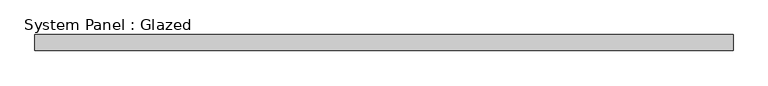
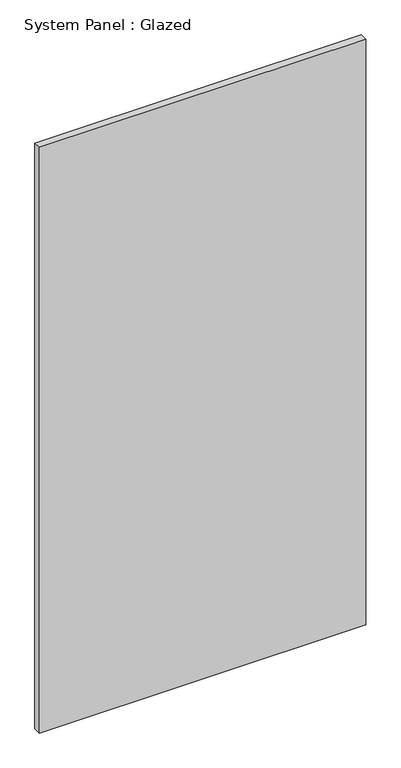
"""IFC4 building model written with IfcOpenShell, lengths in millimetres: plate geometry, System Panel : Glazed."""

from ifc_helpers import new_model, si_unit, origin, origin_with_axes, place, context, project, spatial, polyline, outline, extrude, source, transform, mapped, element, save


def system_panel_glazed_cd98352a(model_context):
    return source(origin(), model_context, "Body", "SweptSolid", [
        extrude(outline(polyline([(555.625, 19.05), (-555.625, 19.05), (-555.625, 44.45), (555.625, 44.45), (555.625, 19.05)])), origin_with_axes(), (0.0, 0.0, 1.0), 2107.5154028),
    ])


if __name__ == "__main__":
    model = new_model("IFC4")
    model_context = context("Model", 3, world=origin())
    ifc_project = project(units=[si_unit("LENGTHUNIT", "METRE", prefix="MILLI")], contexts=[model_context])
    site = spatial("IfcSite", under=ifc_project)
    building = spatial("IfcBuilding", under=site)
    placement = place(None, origin())
    system_panel_glazed_shape = system_panel_glazed_cd98352a(model_context)
    element("IfcPlate", 1, ObjectType="System Panel : Glazed", at=placement, inside=building, context=model_context, shape_type="MappedRepresentation", body=[
        mapped(system_panel_glazed_shape, transform((0.0, 0.0, 0.0), x_axis=(1.0, 0.0, 0.0), y_axis=(0.0, 1.0, 0.0), z_axis=(0.0, 0.0, 1.0))),
    ])
    save(model, "model.ifc")

# Revit data of these elements
# Type "System Panel : Glazed"
#   Construction Type Id = "GSP4R"
#   Analytic Construction = "1/8 in Pilkington single glazing"
#   Visual Light Transmittance = 0.9
#   Solar Heat Gain Coefficient = 0.86
#   Heat Transfer Coefficient (U) = 1.18115 BTU/(h·ft²·°F)
#   Define Thermal Properties by = 1
# Element 1 (IfcPlate, "System Panel : Glazed")
#   Materials on its faces: "Glass"
# Materials
#   "Glass": class "Glass", colour RGB 0 128 192, transparency 0.75, Description = "Soda Lime Glass", Cost = 0
